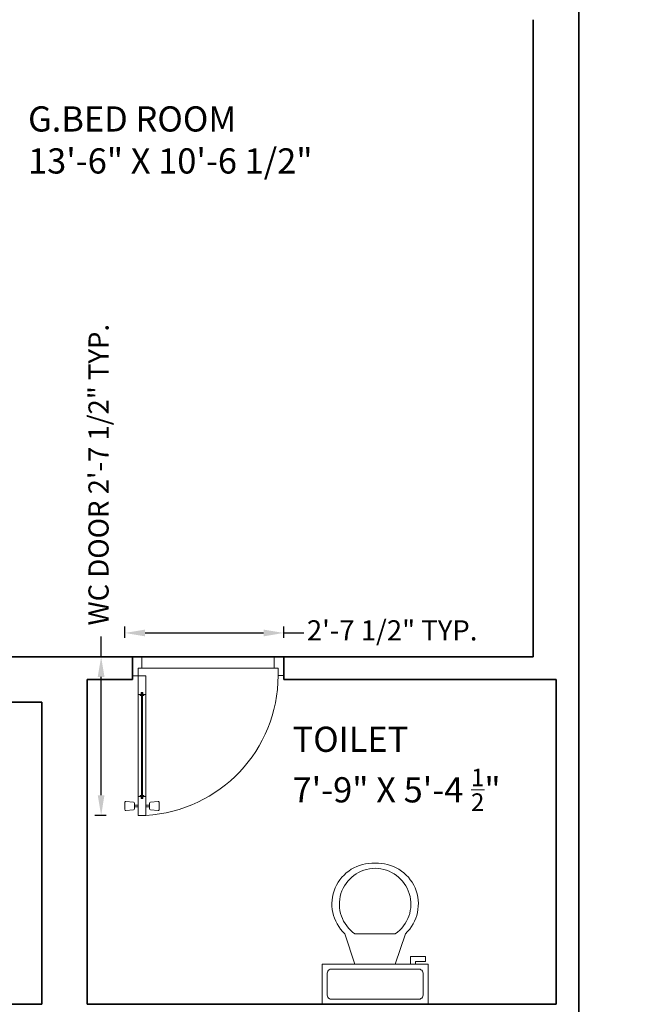
# Model space of a CAD drawing. Units: inches. Extents: x -638 to 186, y -762 to 59.
# Tile 12 of 31: x -100 to 24, y -608 to -413. Entities that reach past the tile are written whole.
import ezdxf

# ---------------------------------------------------------------- set-up
doc = ezdxf.new("R2010")
doc.units = ezdxf.units.IN
for name, color, linetype, lineweight in [('A-ANNO-DIMS', 2, 'Continuous', 18), ('A-AREA-IDEN', 1, 'Continuous', 18), ('A-DOOR', 3, 'Continuous', 18), ('A-FLOR-FIXT', 9, 'Continuous', 18), ('wall', 7, 'Continuous', 35)]:
    doc.layers.add(name, color=color, linetype=linetype, lineweight=lineweight)
doc.styles.get("Standard").update_dxf_attribs({"font": 'arial.ttf'})
doc.dimstyles.new('ISO-25', dxfattribs={"dimtxt": 4, "dimasz": 4, "dimexe": 1.25, "dimexo": 0.625, "dimtad": 0, "dimlunit": 4, "dimtxsty": 'Standard', "dimcen": 2.5, "dimclrt": 256, "dimadec": 0, "dimazin": 0, "dimtfac": 1, "dimtmove": 0, "dimatfit": 3, "dimfxl": 1, "dimfxlon": 1, "dimarcsym": 0})

# ---------------------------------------------------------------- blocks, each defined once
blk = doc.blocks.new('*U4')
for p, q in [((9.5, -6), (9.5, -2)), ((-10, -8.5), (-8, -8.5)), ((-10, -9.5), (-10, -8.5)), ((-7, -9.5), (-10, -9.5)), ((-8, -8.5), (-8, -8)), ((-7, -8), (-7, -9.5)), ((-4, -8), (-6, -14)), ((4, -8), (6, -14)), ((4, -14), (-4, -14))]:
    blk.add_line(p, q)
blk.add_lwpolyline([(10.5, -8), (10.5, 0), (-10.5, 0), (-10.5, -8)], close=True)
for points in [[(8.5, -1), (-8.5, -1)], [(-9.5, -2), (-9.5, -6)], [(-8.5, -7), (8.5, -7)]]:
    blk.add_lwpolyline(points)
for centre, radius, start, end in [((-8.625, -1.875), 0.8839, 81.8699, 188.1301), ((8.625, -1.875), 0.8839, 351.8699, 98.1301), ((-8.625, -6.125), 0.8839, 171.869898, 278.1301), ((8.625, -6.125), 0.8839, 261.8699, 8.1301), ((-0.4772, -19.9188), 8.0953, 133.01722, 273.38), ((0.0374, -19.8731), 7.127, 124.50543, 269.7), ((-0.0373, -19.8731), 7.127, 270.3, 55.4946), ((0.4773, -19.9188), 8.0953, 266.62, 46.9828)]:
    blk.add_arc(centre, radius, start, end)
blk = doc.blocks.new('*D14')
at = {"layer": 'A-ANNO-DIMS', "color": 0, "lineweight": -2, "transparency": 16777216}
for p, q in [((45.41, -42.03), (47.66, -42.03)), ((46.41, -52.03), (46.41, -307.65)), ((46.41, -607.03), (46.41, -351.42)), ((45.41, -617.03), (47.66, -617.03))]:
    blk.add_line(p, q, dxfattribs=at)
at = {"layer": 'A-ANNO-DIMS', "color": 0, "lineweight": 30, "transparency": 16777216}
for points in [[(44.74, -52.03), (48.08, -52.03), (46.41, -42.03)], [(44.74, -607.03), (48.08, -607.03), (46.41, -617.03)]]:
    blk.add_solid(points, dxfattribs=at)
at = {"layer": 'Defpoints', "color": 0, "lineweight": 30, "transparency": 16777216}
for p in [(10.47, -42.03), (10.47, -617.03), (46.41, -617.03)]:
    blk.add_point(p, dxfattribs=at)
at = {"layer": 'A-ANNO-DIMS', "color": 0, "transparency": 16777216, "insert": (46.41, -329.53), "char_height": 10, "attachment_point": 5, "rotation": 90}
blk.add_mtext('47\'-11"', dxfattribs=at)
blk = doc.blocks.new('*D15')
at = {"layer": 'A-ANNO-DIMS', "color": 0, "lineweight": -2, "transparency": 16777216}
for p, q in [((69.33, -24.03), (71.58, -24.03)), ((70.33, -34.03), (70.33, -350.73)), ((70.33, -703.03), (70.33, -386.33)), ((69.33, -713.03), (71.58, -713.03))]:
    blk.add_line(p, q, dxfattribs=at)
at = {"layer": 'A-ANNO-DIMS', "color": 0, "lineweight": 30, "transparency": 16777216}
for points in [[(68.66, -34.03), (72, -34.03), (70.33, -24.03)], [(68.66, -703.03), (72, -703.03), (70.33, -713.03)]]:
    blk.add_solid(points, dxfattribs=at)
at = {"layer": 'Defpoints', "color": 0, "lineweight": 30, "transparency": 16777216}
for p in [(-24.67, -24.03), (-10.56, -713.03), (70.33, -713.03)]:
    blk.add_point(p, dxfattribs=at)
at = {"layer": 'A-ANNO-DIMS', "color": 0, "transparency": 16777216, "insert": (70.33, -368.53), "char_height": 10, "attachment_point": 5, "rotation": 90}
blk.add_mtext('57\'-5"', dxfattribs=at)
blk = doc.blocks.new('DOOR-SWING-30IN')
for p, q in [((29.62, 29.25), (3.38, 29.24)), ((2.64, 3.75), (2.63, 23.99)), ((3.29, 3.37), (3.29, 24.37)), ((3.39, 3.37), (3.38, 24.37)), ((3.48, 3.37), (3.47, 24.37)), ((4.14, 3.75), (4.13, 23.99))]:
    blk.add_line(p, q)
for points in [[(2.63, 27.74), (2.63, 29.24), (3.38, 29.24), (3.38, 31.49), (1.5, 31.49), (1.51, 27.74), (2.63, 27.74)], [(30.37, 27.75), (30.37, 29.25), (29.62, 29.25), (29.62, 31.5), (31.5, 31.5), (31.5, 27.75), (30.37, 27.75)], [(3.57, 23.99), (4.13, 23.99), (4.13, 27.74), (2.63, 27.74), (2.63, 23.99), (3.19, 23.99), (3.19, 24.37), (3.57, 24.37), (3.57, 23.99)], [(3.57, 3.75), (4.14, 3.75), (4.14, 0), (2.64, 0), (2.64, 3.75), (3.2, 3.75), (3.2, 3.37), (3.57, 3.37), (3.57, 3.75)]]:
    blk.add_lwpolyline(points)
for points in [[(1.71, 2.64), (0.21, 2.79, 0.443716), (0, 2.6), (0, 1.14, 0.443716), (0.21, 0.96), (1.71, 1.11, 0.385314), (1.87, 1.29), (1.87, 2.45, 0.385314)], [(5.07, 2.64), (6.57, 2.79, -0.443716), (6.77, 2.61), (6.78, 1.15, -0.443716), (6.57, 0.96), (5.07, 1.11, -0.385314), (4.9, 1.3), (4.9, 2.46, -0.385314)]]:
    blk.add_lwpolyline(points, format="xyb", close=True)
for points in [[(2.64, 2.06), (1.87, 2.06), (1.87, 1.69), (2.64, 1.69)], [(4.14, 2.06), (4.9, 2.06), (4.9, 1.69), (4.14, 1.69)]]:
    blk.add_lwpolyline(points, close=True)
for centre, radius, start, end in [((2.55, 27.77), 27.82, 273.2653, 359.953), ((3.27, 24.03), 0.309, 186.4522, 273.3078), ((3.49, 24.03), 0.309, 266.7282, 353.5838), ((3.28, 3.71), 0.309, 86.7282, 173.5838), ((3.5, 3.71), 0.309, 6.4522, 93.3078)]:
    blk.add_arc(centre, radius, start, end)
blk = doc.blocks.new('*D25')
at = {"layer": 'A-ANNO-DIMS', "color": 0, "lineweight": -2, "transparency": 16777216}
for p, q in [((-84.26, -539.02), (-84.26, -535.02)), ((-83.26, -539.02), (-85.51, -539.02)), ((-84.26, -566.53), (-84.26, -543.02)), ((-83.26, -570.53), (-85.51, -570.53))]:
    blk.add_line(p, q, dxfattribs=at)
at = {"layer": 'A-ANNO-DIMS', "color": 0, "lineweight": 30, "transparency": 16777216}
for points in [[(-84.93, -543.02), (-83.6, -543.02), (-84.26, -539.02)], [(-84.93, -566.53), (-83.6, -566.53), (-84.26, -570.53)]]:
    blk.add_solid(points, dxfattribs=at)
at = {"layer": 'Defpoints', "color": 0, "lineweight": 30, "transparency": 16777216}
for p in [(-84.26, -539.02), (-79.54, -539.02), (-79.54, -570.53)]:
    blk.add_point(p, dxfattribs=at)
at = {"layer": 'A-ANNO-DIMS', "transparency": 16777216, "insert": (-84.26, -502.88), "char_height": 4, "attachment_point": 5, "rotation": 90}
blk.add_mtext('WC DOOR 2\'-7 1/2" TYP.', dxfattribs=at)
blk = doc.blocks.new('*D26')
at = {"layer": 'A-ANNO-DIMS', "color": 0, "lineweight": -2, "transparency": 16777216}
for p, q in [((-79.54, -535.3), (-79.54, -533.05)), ((-48.04, -535.3), (-48.04, -533.05)), ((-75.54, -534.3), (-52.04, -534.3)), ((-48.04, -534.3), (-44.04, -534.3))]:
    blk.add_line(p, q, dxfattribs=at)
at = {"layer": 'A-ANNO-DIMS', "color": 0, "lineweight": 30, "transparency": 16777216}
for points in [[(-75.54, -533.63), (-75.54, -534.97), (-79.54, -534.3)], [(-52.04, -533.63), (-52.04, -534.97), (-48.04, -534.3)]]:
    blk.add_solid(points, dxfattribs=at)
at = {"layer": 'Defpoints', "color": 0, "lineweight": 30, "transparency": 16777216}
for p in [(-48.04, -534.3), (-79.54, -539.02), (-48.04, -539.02)]:
    blk.add_point(p, dxfattribs=at)
at = {"layer": 'A-ANNO-DIMS', "transparency": 16777216, "insert": (-26.53, -534.3), "char_height": 4, "attachment_point": 5}
blk.add_mtext('2\'-7 1/2" TYP.', dxfattribs=at)
blk = doc.blocks.new('*D38')
at = {"layer": 'A-ANNO-DIMS', "color": 0, "lineweight": -2, "transparency": 16777216}
for p, q in [((182.66, -280.53), (184.91, -280.53)), ((183.66, -284.53), (183.66, -371.73)), ((183.66, -473.53), (183.66, -386.34)), ((182.66, -477.53), (184.91, -477.53))]:
    blk.add_line(p, q, dxfattribs=at)
at = {"layer": 'A-ANNO-DIMS', "color": 0, "lineweight": 30, "transparency": 16777216}
for points in [[(183, -284.53), (184.33, -284.53), (183.66, -280.53)], [(183, -473.53), (184.33, -473.53), (183.66, -477.53)]]:
    blk.add_solid(points, dxfattribs=at)
at = {"layer": 'Defpoints', "color": 0, "lineweight": 30, "transparency": 16777216}
for p in [(-404.53, -280.53), (-404.53, -477.53), (183.66, -477.53)]:
    blk.add_point(p, dxfattribs=at)
at = {"layer": 'A-ANNO-DIMS', "transparency": 16777216, "insert": (183.66, -379.03), "char_height": 4, "attachment_point": 5, "rotation": 90}
blk.add_mtext('16\'-5"', dxfattribs=at)
blk = doc.blocks.new('*D52')
at = {"layer": 'A-ANNO-DIMS', "color": 0, "lineweight": -2, "transparency": 16777216}
for p, q in [((-630.93, -580.03), (-633.18, -580.03)), ((-631.93, -584.03), (-631.93, -588.06)), ((-631.93, -604.03), (-631.93, -600.01)), ((-630.93, -608.03), (-633.18, -608.03))]:
    blk.add_line(p, q, dxfattribs=at)
at = {"layer": 'A-ANNO-DIMS', "color": 0, "lineweight": 30, "transparency": 16777216}
for points in [[(-632.59, -584.03), (-631.26, -584.03), (-631.93, -580.03)], [(-632.59, -604.03), (-631.26, -604.03), (-631.93, -608.03)]]:
    blk.add_solid(points, dxfattribs=at)
at = {"layer": 'Defpoints', "color": 0, "lineweight": 30, "transparency": 16777216}
for p in [(-29.91, -580.03), (-631.93, -608.03), (-40.41, -608.03)]:
    blk.add_point(p, dxfattribs=at)
at = {"layer": 'A-ANNO-DIMS', "transparency": 16777216, "insert": (-631.93, -594.03), "char_height": 4, "attachment_point": 5, "rotation": 90}
blk.add_mtext('2\'-4"', dxfattribs=at)

msp = doc.modelspace()

# ---------------------------------------------------------------- linework, layer by layer
at = {"layer": 'wall'}
for p, q in [((10.474, -42.033), (10.474, -617.033)), ((1.474, -412.533), (1.474, -539.033)), ((-160.526, -539.033), (1.474, -539.033)), ((-78.026, -543.533), (-78.026, -539.033)), ((-48.026, -543.533), (-48.026, -539.033)), ((-87.026, -543.533), (-87.026, -608.033)), ((-87.026, -543.533), (-78.026, -543.533)), ((-48.026, -543.533), (5.974, -543.533)), ((5.974, -543.533), (5.974, -608.033)), ((-156.026, -548.033), (-96.026, -548.033)), ((-96.026, -548.033), (-96.026, -608.033)), ((-96.026, -608.033), (-156.026, -608.033)), ((5.974, -608.033), (-87.026, -608.033))]:
    msp.add_line(p, q, dxfattribs=at)

# ---------------------------------------------------------------- block references
at = {"layer": 'A-DOOR'}
msp.add_blockref('DOOR-SWING-30IN', (-79.54, -570.525), dxfattribs=at)
at = {"layer": 'A-FLOR-FIXT', "rotation": 180}
msp.add_blockref('*U4', (-29.908, -608.033), dxfattribs=at)

# ---------------------------------------------------------------- texts
at = {"layer": 'A-AREA-IDEN', "char_height": 5, "attachment_point": 1}
for s, width, insert in [('{G.BED ROOM\\P13\'-6" X 10\'-6 1/2"}', 119.89076, (-98.758, -429.742)), ('\\A1;{TOILET\\P7\'-9" X 5\'-4 \\H0.7x;\\S1/2;\\H1.42857x;"}', 99.04816, (-46.285, -552.91))]:
    msp.add_mtext_dynamic_manual_height_columns(s, width=width, gutter_width=12.5, heights=[0], dxfattribs=dict(at, insert=insert))

# ---------------------------------------------------------------- dimensions: what is measured, and where the dimension line sits
at = {"layer": 'A-ANNO-DIMS'}
for base, p1, p2, override, picture, middle in [((70.331, -713.033), (-24.669, -24.033), (-10.563, -713.033), {"dimtxt": 10, "dimasz": 10, "dimclrd": 0, "dimclre": 0, "dimclrt": 0}, '*D15', (70.331, -368.533)), ((46.411, -617.033), (10.474, -42.033), (10.474, -617.033), {"dimtxt": 10, "dimasz": 10, "dimclrd": 0, "dimclre": 0, "dimclrt": 0}, '*D14', (46.411, -329.533)), ((183.663, -477.533), (-404.526, -280.533), (-404.526, -477.533), {"dimdec": 1, "dimlfac": 1, "dimrnd": 0, "dimzin": 1, "dimdsep": 46, "dimlunit": 4, "dimfrac": 2}, '*D38', (183.663, -379.033)), ((-631.926, -608.033), (-29.908, -580.033), (-40.408, -608.033), {"dimdec": 1, "dimlfac": 1, "dimrnd": 0, "dimzin": 1, "dimdsep": 46, "dimlunit": 4, "dimfrac": 2}, '*D52', (-631.926, -594.033))]:
    dim = msp.add_linear_dim(base=base, p1=p1, p2=p2, angle=90, dimstyle='ISO-25', override=override, dxfattribs=at)
    dim.commit()
    dim.dimension.update_dxf_attribs({"geometry": picture, "text_midpoint": middle})
dim = msp.add_linear_dim(base=(-84.265, -539.024), p1=(-79.54, -570.525), p2=(-79.54, -539.024), angle=90, text='WC DOOR <> TYP.', dimstyle='ISO-25', override={"dimdec": 1, "dimlfac": 1, "dimrnd": 0, "dimzin": 1, "dimdsep": 46, "dimlunit": 4, "dimfrac": 2}, dxfattribs=at)
dim.commit()
dim.dimension.update_dxf_attribs({"geometry": '*D25', "text_midpoint": (-84.265, -502.877)})
dim = msp.add_linear_dim(base=(-48.043, -534.299), p1=(-79.54, -539.024), p2=(-48.043, -539.024), text='<> TYP.', dimstyle='ISO-25', override={"dimdec": 1, "dimlfac": 1, "dimrnd": 0, "dimzin": 1, "dimdsep": 46, "dimlunit": 4, "dimfrac": 2}, dxfattribs=at)
dim.commit()
dim.dimension.update_dxf_attribs({"geometry": '*D26', "text_midpoint": (-26.532, -534.299)})

doc.saveas('drawing.dxf')
